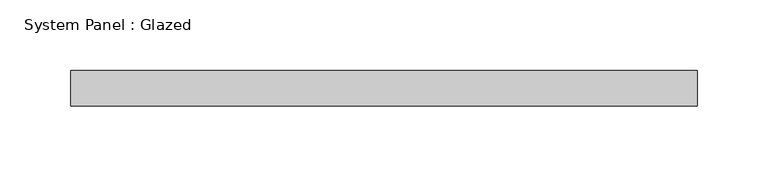
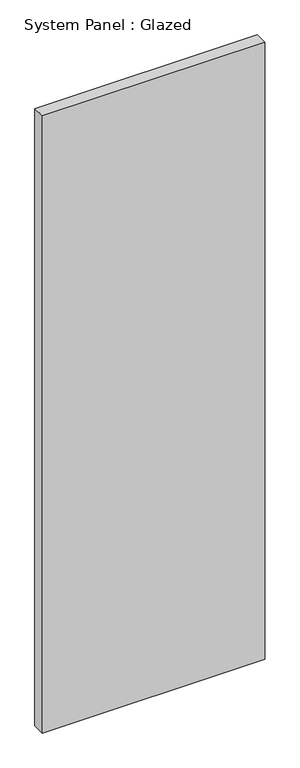
"""IFC4 building model written with IfcOpenShell, lengths in millimetres: plate geometry, System Panel : Glazed."""

from ifc_helpers import new_model, si_unit, origin, origin_with_axes, place, context, project, spatial, polyline, outline, extrude, source, transform, mapped, element, save


def system_panel_glazed_f5573ca5(model_context):
    return source(origin(), model_context, "Body", "SweptSolid", [
        extrude(outline(polyline([(222.25, 19.05), (-222.25, 19.05), (-222.25, 44.45), (222.25, 44.45), (222.25, 19.05)])), origin_with_axes(), (0.0, 0.0, 1.0), 1303.8419021),
    ])


if __name__ == "__main__":
    model = new_model("IFC4")
    model_context = context("Model", 3, world=origin())
    ifc_project = project(units=[si_unit("LENGTHUNIT", "METRE", prefix="MILLI")], contexts=[model_context])
    site = spatial("IfcSite", under=ifc_project)
    building = spatial("IfcBuilding", under=site)
    placement = place(None, origin())
    system_panel_glazed_shape = system_panel_glazed_f5573ca5(model_context)
    element("IfcPlate", 1, ObjectType="System Panel : Glazed", at=placement, inside=building, context=model_context, shape_type="MappedRepresentation", body=[
        mapped(system_panel_glazed_shape, transform((0.0, 0.0, 0.0), x_axis=(1.0, 0.0, 0.0), y_axis=(0.0, 1.0, 0.0), z_axis=(0.0, 0.0, 1.0))),
    ])
    save(model, "model.ifc")

# Revit data of these elements
# Type "System Panel : Glazed"
#   Construction Type Id = "GSP4R"
#   Analytic Construction = "1/8 in Pilkington single glazing"
#   Visual Light Transmittance = 0.9
#   Solar Heat Gain Coefficient = 0.86
#   Heat Transfer Coefficient (U) = 1.18115 BTU/(h·ft²·°F)
#   Define Thermal Properties by = 1
# Element 1 (IfcPlate, "System Panel : Glazed")
#   Materials on its faces: "Glass"
# Materials
#   "Glass": class "Glass", colour RGB 0 128 192, transparency 0.75, Description = "Soda Lime Glass", Cost = 0
